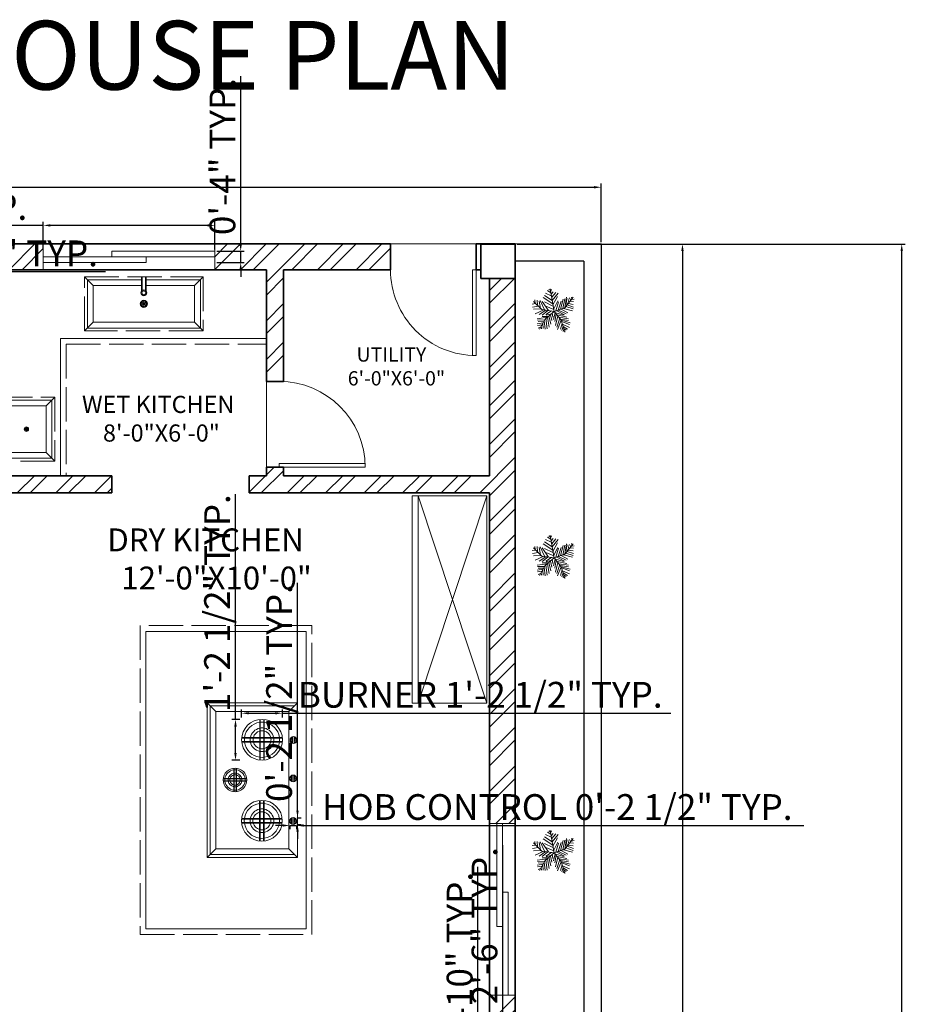
# Model space of a CAD drawing. Units: inches. Extents: x 889 to 1572, y 7262 to 8387.
# Tile 8 of 8: x 1263 to 1572, y 8007 to 8351. Entities that reach past the tile are written whole.
import ezdxf

# ---------------------------------------------------------------- set-up
doc = ezdxf.new("R2010")
doc.units = ezdxf.units.IN
doc.linetypes.add('ACAD_ISO02W100', pattern=[15, 12, -3])
for name, color, linetype, lineweight in [('A-ANNO-DIMS', 2, 'Continuous', 18), ('A-ANNO-TITL', 7, 'Continuous', 35), ('A-AREA-IDEN', 7, 'Continuous', 18), ('A-CASE-HIDN', 8, 'ACAD_ISO02W100', 13), ('A-DOOR', 4, 'Continuous', 18), ('A-EQPM', 8, 'Continuous', 18), ('A-FIXT-HIDN', 9, 'ACAD_ISO02W100', 13), ('A-FLOR-CASE', 8, 'Continuous', 20), ('A-FLOR-FIXT', 9, 'Continuous', 18), ('A-WALL', 7, 'Continuous', 35), ('A-WALL-PATT', 252, 'Continuous', 13), ('C-SITE', 7, 'Continuous', 30), ('L-PLNT', 94, 'Continuous', 13)]:
    doc.layers.add(name, color=color, linetype=linetype, lineweight=lineweight)
doc.layers.add('A-GLAZ', color=244, linetype='Continuous', lineweight=18, true_color=0x991b1e)
doc.styles.get("Standard").update_dxf_attribs({"font": 'arial.ttf'})
doc.dimstyles.new('ISO-25', dxfattribs={"dimtxt": 9, "dimasz": 2.5, "dimexe": 1.25, "dimexo": 0.625, "dimtad": 1, "dimlunit": 3, "dimtxsty": 'Standard', "dimcen": 2.5, "dimadec": 0, "dimazin": 0, "dimtfac": 1, "dimtmove": 0, "dimatfit": 3, "dimfxl": 1, "dimarcsym": 0})

# ---------------------------------------------------------------- blocks, each defined once
blk = doc.blocks.new('*U3')
for p, q in [((0, 0), (0, -6)), ((-40, 0), (-40, -6))]:
    blk.add_line(p, q)
blk.add_lwpolyline([(0, 0), (0, 40), (-1.75, 40), (-1.75, 0)], close=True)
blk.add_arc((0, 0), 40, 90, 180)
blk = doc.blocks.new('*U8')
for p, q in [((0, 0), (0, -6)), ((40, 0), (40, -6))]:
    blk.add_line(p, q)
blk.add_lwpolyline([(0, 0), (0, 40), (1.75, 40), (1.75, 0)], close=True)
blk.add_arc((0, 0), 40, 0, 90)
blk = doc.blocks.new('*U15')
for p, q in [((-8.737, 47.138), (-17.069, 52.711)), ((-10.186, 53.64), (-13.084, 55.962)), ((0, 0), (-10.5, 57)), ((-9.099, 51.782), (-6.563, 55.962)), ((-31.5, 4.5), (-52.5, 25.5)), ((-48.585, 21.131), (-49.309, 29.026)), ((-43.513, 28.561), (-42.427, 15.558)), ((-38.442, 26.239), (-34.819, 7.663)), ((-35.544, 28.097), (-24.314, 3.947)), ((-14.533, 2.09), (-30.834, 25.31)), ((-3.665, 19.273), (-27.574, 35.527)), ((-5.114, 28.097), (-24.676, 40.636)), ((-7.288, 39.707), (-21.778, 46.673)), ((-7.65, 43.423), (-2.578, 49.46)), ((-5.839, 35.992), (4.667, 48.067)), ((-5.114, 27.632), (10.463, 46.673)), ((-2.941, 16.486), (8.652, 37.85)), ((-1.129, 6.734), (9.014, 26.704)), ((10.101, 3.483), (17.708, 26.239)), ((16.259, 5.805), (23.142, 31.348)), ((22.055, 7.198), (27.489, 32.277)), ((27, 9), (48, 36)), ((27.127, 9.056), (31.112, 35.992)), ((31.836, 30.883), (32.561, 16.486)), ((35.096, 32.741), (37.27, 22.524)), ((38.719, 34.134), (41.979, 28.561)), ((40.53, 25.775), (48.862, 24.846)), ((43.791, 29.954), (51.036, 30.883)), ((44.153, 36.456), (45.239, 32.741)), ((-47.498, 19.737), (-55.83, 18.344)), ((-40.615, 13.7), (-55.105, 10.913)), ((-33.37, 6.269), (-52.207, 5.34)), ((-28.299, 3.483), (-47.86, -5.805)), ((-21.416, 3.018), (-38.079, -8.128)), ((0, 0), (-31.5, 4.5)), ((-15.982, 2.09), (-30.11, -9.521)), ((-24.314, 23.917), (-2.941, 13.7)), ((0, 0), (-22.5, -19.5)), ((-6.563, 1.161), (-21.416, -8.128)), ((-20.691, 13.7), (-1.129, 4.876)), ((0, 0), (27, 9)), ((0, 0), (18, -22.5)), ((3.942, 1.625), (11.187, 24.381)), ((6.478, 1.625), (26.04, -8.592)), ((11.187, 3.483), (30.749, -5.805)), ((18.07, 5.805), (35.096, -3.483)), ((24.229, 7.663), (46.688, 1.625)), ((29.662, 12.307), (48.137, 6.269)), ((33.285, 16.486), (48.862, 10.913)), ((36.183, 19.737), (48.137, 17.88)), ((-17.431, -15.094), (-42.789, -18.809)), ((-24.314, -21.596), (-42.427, -22.06)), ((-22.5, -19.5), (-37.5, -45)), ((-15.257, -12.772), (-30.11, -12.772)), ((-25.038, -23.918), (-22.865, -45.281)), ((-20.691, -18.345), (-17.793, -44.352)), ((-6.563, -5.805), (-19.967, -9.985)), ((-17.069, -15.094), (-12.721, -40.172)), ((-13.446, -11.378), (-8.737, -32.741)), ((-9.461, -8.592), (-6.201, -23.453)), ((-4.752, -3.483), (-3.665, -14.629)), ((2.493, -3.019), (-1.491, -20.202)), ((1.769, -2.555), (24.229, -9.521)), ((5.029, -6.27), (2.131, -25.775)), ((9.014, -11.378), (3.58, -35.992)), ((14.085, -16.951), (6.478, -40.172)), ((7.565, -9.056), (32.198, -14.629)), ((18.07, -22.524), (8.289, -45.745)), ((12.274, -15.094), (36.907, -18.809)), ((16.259, -19.738), (36.183, -22.989)), ((18, -22.5), (27, -52.5)), ((18.433, -22.524), (40.53, -29.026)), ((-28.299, -29.026), (-42.789, -31.348)), ((-30.834, -34.135), (-42.427, -35.528)), ((-34.457, -39.708), (-40.978, -42.494)), ((-26.849, -26.24), (-40.253, -25.775)), ((-32.646, -36.921), (-31.921, -44.352)), ((-29.023, -30.884), (-27.936, -43.887)), ((20.244, -30.419), (15.897, -44.816)), ((19.157, -25.311), (38.719, -33.206)), ((22.78, -37.85), (19.519, -48.532)), ((21.331, -32.741), (39.081, -40.636)), ((22.78, -38.314), (34.372, -44.816)), ((24.591, -45.745), (23.142, -50.854)), ((24.591, -43.423), (30.749, -47.603)), ((26.764, -49.925), (28.213, -50.854))]:
    blk.add_line(p, q)
blk = doc.blocks.new('*D28')
at = {"layer": 'A-ANNO-DIMS', "color": 0, "lineweight": -2, "transparency": 16777216}
for p, q in [((986.05, 8273.36), (986.05, 8293.82)), ((1466.05, 8273.36), (1466.05, 8293.82)), ((988.55, 8292.57), (1463.55, 8292.57))]:
    blk.add_line(p, q, dxfattribs=at)
at = {"layer": 'A-ANNO-DIMS', "color": 0, "transparency": 16777216}
for points in [[(988.55, 8292.98), (988.55, 8292.15), (986.05, 8292.57)], [(1463.55, 8292.98), (1463.55, 8292.15), (1466.05, 8292.57)]]:
    blk.add_solid(points, dxfattribs=at)
at = {"layer": 'Defpoints', "color": 0, "transparency": 16777216}
for p in [(1466.05, 8292.57), (986.05, 8272.73), (1466.05, 8272.73)]:
    blk.add_point(p, dxfattribs=at)
at = {"layer": 'A-ANNO-DIMS', "color": 0, "transparency": 16777216, "insert": (1226.05, 8297.79), "char_height": 9, "attachment_point": 5}
blk.add_mtext("40'", dxfattribs=at)
blk = doc.blocks.new('*D29')
at = {"layer": 'A-ANNO-DIMS', "color": 0, "lineweight": -2, "transparency": 16777216}
for p, q in [((1466.67, 8272.73), (1495.73, 8272.73)), ((1494.48, 8270.23), (1494.48, 7396.23)), ((1466.67, 7393.73), (1495.73, 7393.73))]:
    blk.add_line(p, q, dxfattribs=at)
at = {"layer": 'A-ANNO-DIMS', "color": 0, "transparency": 16777216}
for points in [[(1494.06, 8270.23), (1494.9, 8270.23), (1494.48, 8272.73)], [(1494.06, 7396.23), (1494.9, 7396.23), (1494.48, 7393.73)]]:
    blk.add_solid(points, dxfattribs=at)
at = {"layer": 'Defpoints', "color": 0, "transparency": 16777216}
for p in [(1466.05, 8272.73), (1466.05, 7393.73), (1494.48, 7393.73)]:
    blk.add_point(p, dxfattribs=at)
at = {"layer": 'A-ANNO-DIMS', "color": 0, "transparency": 16777216, "insert": (1489.26, 7833.23), "char_height": 9, "attachment_point": 5, "rotation": 90}
blk.add_mtext('73\'-3"', dxfattribs=at)
blk = doc.blocks.new('COOKTOP-BURNER-LARGE')
for p, q in [((6.34, 14.23), (6.34, 0.05)), ((6.54, 14.25), (6.54, 7.94)), ((7.74, 14.25), (7.74, 7.94)), ((7.94, 14.23), (7.94, 0.05)), ((0.03, 7.74), (6.34, 7.74)), ((0.05, 7.94), (14.23, 7.94)), ((6.54, 7.74), (6.54, 6.54)), ((6.54, 7.74), (7.74, 7.74)), ((7.74, 7.74), (7.74, 6.54)), ((7.94, 7.74), (14.25, 7.74)), ((0.03, 6.54), (6.34, 6.54)), ((0.05, 6.34), (14.23, 6.34)), ((6.54, 6.54), (7.74, 6.54)), ((6.54, 6.34), (6.54, 0.03)), ((7.74, 6.34), (7.74, 0.03)), ((7.94, 6.54), (14.25, 6.54))]:
    blk.add_line(p, q)
blk.add_circle((7.14, 7.14), 7.14)
for radius, start, end in [(6.14, 97.4895, 172.5105), (4.14, 101.1483, 168.8517), (6.14, 84.3899, 95.6101), (4.14, 81.662, 98.338), (6.14, 7.4895, 82.5105), (4.14, 11.1483, 78.8517), (6.14, 174.3899, 185.6101), (4.14, 171.662, 188.338), (3.14, 168.9754, 191.0246), (3.14, 104.772, 165.228), (3.14, 78.9754, 101.0246), (3.14, 14.772, 75.228), (3.14, 348.9754, 11.0246), (4.14, 351.662, 8.338), (6.14, 354.3899, 5.6101), (6.14, 187.4895, 262.5105), (4.14, 191.1483, 258.8517), (3.14, 194.772, 255.228), (3.14, 258.9754, 281.0246), (3.14, 284.772, 345.228), (4.14, 281.1483, 348.8517), (6.14, 277.4895, 352.5105), (4.14, 261.662, 278.338), (6.14, 264.3899, 275.6101)]:
    blk.add_arc((7.14, 7.14), radius, start, end)
blk = doc.blocks.new('COOKTOP-CONTROL')
for p, q in [((0.89, 2.34), (0.89, 0.04)), ((1.49, 2.34), (1.49, 0.04))]:
    blk.add_line(p, q)
blk.add_circle((1.19, 1.19), 1.19)
for radius, start, end in [(0.987, 107.6863, 252.3137), (0.587, 120.7077, 239.2923), (0.387, 140.7361, 219.2639), (0.987, 287.6863, 72.3137), (0.587, 300.7077, 59.2923), (0.387, 320.7361, 39.2639)]:
    blk.add_arc((1.19, 1.19), radius, start, end)
blk = doc.blocks.new('GLAZ-SLIDER-60IN')
for p, q in [((0, 60), (0, 24)), ((2, 60), (2, 0)), ((2, 36), (4, 36)), ((4, 36), (4, 0)), ((2, 24), (0, 24))]:
    blk.add_line(p, q)
blk = doc.blocks.new('*D37')
at = {"layer": 'A-ANNO-DIMS', "color": 0, "lineweight": -2, "transparency": 16777216}
for p, q in [((1271.05, 8279.23), (1163.57, 8279.23)), ((1271.05, 8270.86), (1271.05, 8280.48)), ((1328.55, 8279.23), (1273.55, 8279.23)), ((1331.05, 8270.86), (1331.05, 8280.48))]:
    blk.add_line(p, q, dxfattribs=at)
at = {"layer": 'A-ANNO-DIMS', "color": 0, "transparency": 16777216}
for points in [[(1273.55, 8279.65), (1273.55, 8278.81), (1271.05, 8279.23)], [(1328.55, 8279.65), (1328.55, 8278.81), (1331.05, 8279.23)]]:
    blk.add_solid(points, dxfattribs=at)
at = {"layer": 'Defpoints', "color": 0, "transparency": 16777216}
for p in [(1271.05, 8279.23), (1271.05, 8270.23), (1331.05, 8270.23)]:
    blk.add_point(p, dxfattribs=at)
at = {"layer": 'A-ANNO-DIMS', "color": 0, "transparency": 16777216, "insert": (1216.06, 8284.51), "char_height": 9, "attachment_point": 5}
blk.add_mtext('SLIDER 5\'-0" TYP.', dxfattribs=at)
blk = doc.blocks.new('*D38')
at = {"layer": 'A-ANNO-DIMS', "color": 0, "lineweight": -2, "transparency": 16777216}
for p, q in [((1340.05, 8272.73), (1340.05, 8331.34)), ((1331.67, 8270.23), (1341.3, 8270.23)), ((1340.05, 8266.23), (1340.05, 8270.23)), ((1331.67, 8266.23), (1341.3, 8266.23)), ((1340.05, 8263.73), (1340.05, 8261.23))]:
    blk.add_line(p, q, dxfattribs=at)
at = {"layer": 'A-ANNO-DIMS', "color": 0, "transparency": 16777216}
for points in [[(1339.63, 8272.73), (1340.47, 8272.73), (1340.05, 8270.23)], [(1339.63, 8263.73), (1340.47, 8263.73), (1340.05, 8266.23)]]:
    blk.add_solid(points, dxfattribs=at)
at = {"layer": 'Defpoints', "color": 0, "transparency": 16777216}
for p in [(1331.05, 8270.23), (1340.05, 8270.23), (1331.05, 8266.23)]:
    blk.add_point(p, dxfattribs=at)
at = {"layer": 'A-ANNO-DIMS', "color": 0, "transparency": 16777216, "insert": (1334.83, 8303.29), "char_height": 9, "attachment_point": 5, "rotation": 90}
blk.add_mtext('0\'-4" TYP.', dxfattribs=at)
blk = doc.blocks.new('*D41')
at = {"layer": 'A-ANNO-DIMS', "color": 0, "lineweight": -2, "transparency": 16777216}
for p, q in [((1175.74, 8265.61), (1175.74, 8261.83)), ((1196.74, 8265.61), (1196.74, 8261.83)), ((1178.24, 8263.08), (1194.24, 8263.08)), ((1196.74, 8263.08), (1292.84, 8263.08))]:
    blk.add_line(p, q, dxfattribs=at)
at = {"layer": 'A-ANNO-DIMS', "color": 0, "transparency": 16777216}
for points in [[(1178.24, 8263.5), (1178.24, 8262.66), (1175.74, 8263.08)], [(1194.24, 8263.5), (1194.24, 8262.66), (1196.74, 8263.08)]]:
    blk.add_solid(points, dxfattribs=at)
at = {"layer": 'Defpoints', "color": 0, "transparency": 16777216}
for p in [(1175.74, 8266.23), (1196.74, 8266.23), (1196.74, 8263.08)]:
    blk.add_point(p, dxfattribs=at)
at = {"layer": 'A-ANNO-DIMS', "color": 0, "transparency": 16777216, "insert": (1246.04, 8268.3), "char_height": 9, "attachment_point": 5}
blk.add_mtext('VENT 1\'-9" TYP.', dxfattribs=at)
blk = doc.blocks.new('*D48')
at = {"layer": 'A-ANNO-DIMS', "color": 0, "lineweight": -2, "transparency": 16777216}
for p, q in [((1431.66, 8003.87), (1431.66, 8062.63)), ((1426.67, 8003.87), (1432.91, 8003.87)), ((1431.66, 7976.19), (1431.66, 8001.37)), ((1426.67, 7973.69), (1432.91, 7973.69))]:
    blk.add_line(p, q, dxfattribs=at)
at = {"layer": 'A-ANNO-DIMS', "color": 0, "transparency": 16777216}
for points in [[(1431.24, 8001.37), (1432.07, 8001.37), (1431.66, 8003.87)], [(1431.24, 7976.19), (1432.07, 7976.19), (1431.66, 7973.69)]]:
    blk.add_solid(points, dxfattribs=at)
at = {"layer": 'Defpoints', "color": 0, "transparency": 16777216}
for p in [(1426.05, 8003.87), (1431.66, 8003.87), (1426.05, 7973.69)]:
    blk.add_point(p, dxfattribs=at)
at = {"layer": 'A-ANNO-DIMS', "color": 0, "transparency": 16777216, "insert": (1426.44, 8034.5), "char_height": 9, "attachment_point": 5, "rotation": 90}
blk.add_mtext('2\'-6" TYP.', dxfattribs=at)
blk = doc.blocks.new('*D55')
at = {"layer": 'A-ANNO-DIMS', "color": 0, "lineweight": -2, "transparency": 16777216}
for p, q in [((1354.69, 8069.51), (1352.19, 8069.51)), ((1357.19, 8069.51), (1359.56, 8069.51)), ((1357.19, 8069.25), (1357.19, 8068.26)), ((1359.56, 8069.25), (1359.56, 8068.26)), ((1362.06, 8069.51), (1536.86, 8069.51))]:
    blk.add_line(p, q, dxfattribs=at)
at = {"layer": 'A-ANNO-DIMS', "color": 0, "transparency": 16777216}
for points in [[(1354.69, 8069.93), (1354.69, 8069.1), (1357.19, 8069.51)], [(1362.06, 8069.93), (1362.06, 8069.1), (1359.56, 8069.51)]]:
    blk.add_solid(points, dxfattribs=at)
at = {"layer": 'Defpoints', "color": 0, "transparency": 16777216}
for p in [(1357.19, 8069.87), (1359.56, 8069.87), (1359.56, 8069.51)]:
    blk.add_point(p, dxfattribs=at)
at = {"layer": 'A-ANNO-DIMS', "color": 0, "transparency": 16777216, "insert": (1450.71, 8074.8), "char_height": 9, "attachment_point": 5}
blk.add_mtext('HOB CONTROL 0\'-2 1/2" TYP.', dxfattribs=at)
blk = doc.blocks.new('*D56')
at = {"layer": 'A-ANNO-DIMS', "color": 0, "lineweight": -2, "transparency": 16777216}
for p, q in [((1359.92, 8074.75), (1359.92, 8154.33)), ((1359.92, 8069.87), (1359.92, 8072.25)), ((1360.19, 8072.25), (1361.17, 8072.25)), ((1360.19, 8069.87), (1361.17, 8069.87)), ((1359.92, 8067.37), (1359.92, 8064.87))]:
    blk.add_line(p, q, dxfattribs=at)
at = {"layer": 'A-ANNO-DIMS', "color": 0, "transparency": 16777216}
for points in [[(1359.5, 8074.75), (1360.33, 8074.75), (1359.92, 8072.25)], [(1359.5, 8067.37), (1360.33, 8067.37), (1359.92, 8069.87)]]:
    blk.add_solid(points, dxfattribs=at)
at = {"layer": 'Defpoints', "color": 0, "transparency": 16777216}
for p in [(1359.56, 8072.25), (1359.56, 8069.87), (1359.92, 8072.25)]:
    blk.add_point(p, dxfattribs=at)
at = {"layer": 'A-ANNO-DIMS', "color": 0, "transparency": 16777216, "insert": (1354.64, 8115.79), "char_height": 9, "attachment_point": 5, "rotation": 90}
blk.add_mtext('0\'-2 1/2" TYP.', dxfattribs=at)
blk = doc.blocks.new('*D57')
at = {"layer": 'A-ANNO-DIMS', "color": 0, "lineweight": -2, "transparency": 16777216}
for p, q in [((1422.97, 7957.73), (1422.97, 8055.08)), ((1418.49, 7957.73), (1424.22, 7957.73)), ((1422.97, 7926.23), (1422.97, 7955.23)), ((1418.49, 7923.73), (1424.22, 7923.73))]:
    blk.add_line(p, q, dxfattribs=at)
at = {"layer": 'A-ANNO-DIMS', "color": 0, "transparency": 16777216}
for points in [[(1422.55, 7955.23), (1423.38, 7955.23), (1422.97, 7957.73)], [(1422.55, 7926.23), (1423.38, 7926.23), (1422.97, 7923.73)]]:
    blk.add_solid(points, dxfattribs=at)
at = {"layer": 'Defpoints', "color": 0, "transparency": 16777216}
for p in [(1417.87, 7957.73), (1422.97, 7957.73), (1417.87, 7923.73)]:
    blk.add_point(p, dxfattribs=at)
at = {"layer": 'A-ANNO-DIMS', "color": 0, "transparency": 16777216, "insert": (1417.74, 8007.65), "char_height": 9, "attachment_point": 5, "rotation": 90}
blk.add_mtext('BIKE 2\'-10" TYP.', dxfattribs=at)
blk = doc.blocks.new('*D61')
at = {"layer": 'A-ANNO-DIMS', "color": 0, "lineweight": -2, "transparency": 16777216}
for p, q in [((1340.38, 8107.23), (1340.38, 8110)), ((1342.88, 8108.75), (1352.15, 8108.75)), ((1354.65, 8107.23), (1354.65, 8110)), ((1354.65, 8108.75), (1490.42, 8108.75))]:
    blk.add_line(p, q, dxfattribs=at)
at = {"layer": 'A-ANNO-DIMS', "color": 0, "transparency": 16777216}
for points in [[(1342.88, 8109.16), (1342.88, 8108.33), (1340.38, 8108.75)], [(1352.15, 8109.16), (1352.15, 8108.33), (1354.65, 8108.75)]]:
    blk.add_solid(points, dxfattribs=at)
at = {"layer": 'Defpoints', "color": 0, "transparency": 16777216}
for p in [(1354.65, 8108.75), (1340.38, 8106.61), (1354.65, 8106.61)]:
    blk.add_point(p, dxfattribs=at)
at = {"layer": 'A-ANNO-DIMS', "color": 0, "transparency": 16777216, "insert": (1423.78, 8114.03), "char_height": 9, "attachment_point": 5}
blk.add_mtext('BURNER 1\'-2 1/2" TYP.', dxfattribs=at)
blk = doc.blocks.new('*D62')
at = {"layer": 'A-ANNO-DIMS', "color": 0, "lineweight": -2, "transparency": 16777216}
for p, q in [((1338.24, 8106.61), (1338.24, 8185.34)), ((1339.75, 8106.61), (1336.99, 8106.61)), ((1338.24, 8094.83), (1338.24, 8104.11)), ((1339.75, 8092.33), (1336.99, 8092.33))]:
    blk.add_line(p, q, dxfattribs=at)
at = {"layer": 'A-ANNO-DIMS', "color": 0, "transparency": 16777216}
for points in [[(1337.82, 8104.11), (1338.65, 8104.11), (1338.24, 8106.61)], [(1337.82, 8094.83), (1338.65, 8094.83), (1338.24, 8092.33)]]:
    blk.add_solid(points, dxfattribs=at)
at = {"layer": 'Defpoints', "color": 0, "transparency": 16777216}
for p in [(1338.24, 8106.61), (1340.38, 8106.61), (1340.38, 8092.33)]:
    blk.add_point(p, dxfattribs=at)
at = {"layer": 'A-ANNO-DIMS', "color": 0, "transparency": 16777216, "insert": (1332.96, 8147.22), "char_height": 9, "attachment_point": 5, "rotation": 90}
blk.add_mtext('1\'-2 1/2" TYP.', dxfattribs=at)
blk = doc.blocks.new('*D70')
at = {"layer": 'A-ANNO-DIMS', "color": 0, "lineweight": -2, "transparency": 16777216}
for p, q in [((1436.67, 8272.73), (1572.38, 8272.73)), ((1571.13, 7585.23), (1571.13, 8270.23)), ((1436.67, 7582.73), (1572.38, 7582.73))]:
    blk.add_line(p, q, dxfattribs=at)
at = {"layer": 'A-ANNO-DIMS', "color": 0, "transparency": 16777216}
for points in [[(1570.71, 8270.23), (1571.54, 8270.23), (1571.13, 8272.73)], [(1570.71, 7585.23), (1571.54, 7585.23), (1571.13, 7582.73)]]:
    blk.add_solid(points, dxfattribs=at)
at = {"layer": 'Defpoints', "color": 0, "transparency": 16777216}
for p in [(1436.05, 8272.73), (1571.13, 8272.73), (1436.05, 7582.73)]:
    blk.add_point(p, dxfattribs=at)
at = {"layer": 'A-ANNO-DIMS', "color": 0, "transparency": 16777216, "insert": (1565.91, 7927.73), "char_height": 9, "attachment_point": 5, "rotation": 90}
blk.add_mtext('57\'-6"', dxfattribs=at)
blk = doc.blocks.new('*D74')
at = {"layer": 'A-ANNO-DIMS', "color": 0, "lineweight": -2, "transparency": 16777216}
for p, q in [((1247.05, 8161.11), (1247.05, 7262.35)), ((1253.05, 8161.11), (1253.05, 7262.35)), ((1244.55, 7263.6), (1242.05, 7263.6)), ((1247.05, 7263.6), (1253.05, 7263.6)), ((1255.55, 7263.6), (1283.22, 7263.6))]:
    blk.add_line(p, q, dxfattribs=at)
at = {"layer": 'A-ANNO-DIMS', "color": 0, "transparency": 16777216}
for points in [[(1244.55, 7264.02), (1244.55, 7263.19), (1247.05, 7263.6)], [(1255.55, 7264.02), (1255.55, 7263.19), (1253.05, 7263.6)]]:
    blk.add_solid(points, dxfattribs=at)
at = {"layer": 'Defpoints', "color": 0, "transparency": 16777216}
for p in [(1247.05, 8161.73), (1253.05, 8161.73), (1253.05, 7263.6)]:
    blk.add_point(p, dxfattribs=at)
at = {"layer": 'A-ANNO-DIMS', "color": 0, "transparency": 16777216, "insert": (1270.64, 7268.82), "char_height": 9, "attachment_point": 5}
blk.add_mtext('0\'-6"', dxfattribs=at)

msp = doc.modelspace()

# ---------------------------------------------------------------- hatches: boundary and pattern name
at = {"layer": 'A-WALL-PATT'}
h = msp.add_hatch(dxfattribs=at)
h.set_pattern_fill('ANSI32', color=256)
h.paths.add_polyline_path([(1166.049, 7624.731), (1163.049, 7624.731), (1163.049, 7774.731), (1154.049, 7774.731), (1154.049, 7768.731), (1157.049, 7768.731), (1157.049, 7624.731), (1106.049, 7624.731), (1106.049, 7615.731), (1166.049, 7615.731), (1166.049, 7618.431)])
h.paths.add_polyline_path([(1025.049, 7666.731), (1016.049, 7666.731), (1016.049, 7615.731), (1076.049, 7615.731), (1076.049, 7624.731), (1025.049, 7624.731)])
h.paths.add_polyline_path([(1025.049, 7768.731), (1118.049, 7768.731), (1118.049, 7774.731), (1025.049, 7774.731), (1025.049, 7897.731), (1115.049, 7897.731), (1115.049, 7906.731), (1109.049, 7906.731), (1109.049, 7903.731), (1025.049, 7903.731), (1025.049, 7923.231), (1016.049, 7923.231), (1016.049, 7726.731), (1025.049, 7726.731)])
h.paths.add_polyline_path([(1436.049, 7897.731), (1427.049, 7897.731), (1427.049, 7883.374), (1436.049, 7883.374)])
h.paths.add_polyline_path([(1436.049, 7853.374), (1427.049, 7853.374), (1427.049, 7843.731), (1415.049, 7843.731), (1415.049, 7837.731), (1427.049, 7837.731), (1427.049, 7831.731), (1436.049, 7831.731)])
h.paths.add_polyline_path([(1436.049, 8010.183), (1427.049, 8010.183), (1427.049, 7970.456), (1370.049, 7970.456), (1370.049, 7963.731), (1427.049, 7963.731), (1427.049, 7957.731), (1436.049, 7957.731)])
h.paths.add_polyline_path([(1436.049, 7747.731), (1427.049, 7747.731), (1427.049, 7741.731), (1344.721, 7741.731), (1344.721, 7735.731), (1349.049, 7735.731), (1349.049, 7672.731), (1355.049, 7672.731), (1355.049, 7735.731), (1427.049, 7735.731), (1427.049, 7721.931), (1436.049, 7721.931)])
h.paths.add_polyline_path([(1436.049, 7700.931), (1427.049, 7700.931), (1427.049, 7591.731), (1355.049, 7591.731), (1355.049, 7642.731), (1349.049, 7642.731), (1349.049, 7591.731), (1310.049, 7591.731), (1310.049, 7582.731), (1436.049, 7582.731)])
h.paths.add_polyline_path([(1392.42, 8272.731), (1331.049, 8272.731), (1331.049, 8263.731), (1349.049, 8263.731), (1349.049, 8224.731), (1355.049, 8224.731), (1355.049, 8263.731), (1392.42, 8263.731)])
h.paths.add_polyline_path([(1271.049, 8272.731), (1196.736, 8272.731), (1196.736, 8263.731), (1247.049, 8263.731), (1247.049, 8203.731), (1244.049, 8203.731), (1244.049, 8197.731), (1247.049, 8197.731), (1247.049, 8161.731), (1253.049, 8161.731), (1253.049, 8185.731), (1295.049, 8185.731), (1295.049, 8191.731), (1253.049, 8191.731), (1253.049, 8263.731), (1271.049, 8263.731)])
h.paths.add_polyline_path([(1175.736, 8272.731), (1102.037, 8272.731), (1102.037, 8263.731), (1157.049, 8263.731), (1157.049, 8158.731), (1163.049, 8158.731), (1163.049, 8197.731), (1214.049, 8197.731), (1214.049, 8203.731), (1163.049, 8203.731), (1163.049, 8263.731), (1175.736, 8263.731)])
h.paths.add_polyline_path([(1072.037, 8272.731), (1016.049, 8272.731), (1016.049, 8221.731), (1025.049, 8221.731), (1025.049, 8263.731), (1072.037, 8263.731)])
h.paths.add_polyline_path([(1163.049, 8122.731), (1157.049, 8122.731), (1157.049, 8119.731), (1025.049, 8119.731), (1025.049, 8161.731), (1016.049, 8161.731), (1016.049, 8071.731), (1025.049, 8071.731), (1025.049, 8113.731), (1157.049, 8113.731), (1157.049, 8110.731), (1163.049, 8110.731)])
h.paths.add_polyline_path([(1025.049, 8011.731), (1016.049, 8011.731), (1016.049, 7944.231), (1025.049, 7944.231), (1025.049, 7963.731), (1109.049, 7963.731), (1109.049, 7936.731), (1115.049, 7936.731), (1115.049, 7963.731), (1163.049, 7963.731), (1163.049, 8074.731), (1157.049, 8074.731), (1157.049, 7969.731), (1025.049, 7969.731)])
h.paths.add_polyline_path([(1314.721, 7741.731), (1307.049, 7741.731), (1307.049, 7837.731), (1319.049, 7837.731), (1319.049, 7843.731), (1307.049, 7843.731), (1307.049, 7963.731), (1310.049, 7963.731), (1310.049, 7970.456), (1301.049, 7970.456), (1301.049, 7837.731), (1301.049, 7741.731), (1250.049, 7741.731), (1250.049, 7735.731), (1314.721, 7735.731)])
h.paths.add_polyline_path([(1211.049, 7735.731), (1214.049, 7735.731), (1214.049, 7741.731), (1205.049, 7741.731), (1205.049, 7624.731), (1202.049, 7624.731), (1202.049, 7615.731), (1205.049, 7615.731), (1205.049, 7582.731), (1250.049, 7582.731), (1250.049, 7591.731), (1211.049, 7591.731)])
h.paths.add_polyline_path([(1436.049, 8260.718), (1427.049, 8260.718), (1427.049, 8191.731), (1355.049, 8191.731), (1355.049, 8194.731), (1349.049, 8194.731), (1349.049, 8191.731), (1343.049, 8191.731), (1343.049, 8185.731), (1427.049, 8185.731), (1427.049, 8070.183), (1436.049, 8070.183)])

# ---------------------------------------------------------------- linework, layer by layer
at = {"layer": 'A-CASE-HIDN'}
for q in [(1349.049, 8237.731), (1279.049, 8191.731)]:
    msp.add_line((1279.049, 8237.731), q, dxfattribs=at)
msp.add_lwpolyline([(1364.909, 8139.364), (1304.909, 8139.364), (1304.909, 8031.364), (1364.909, 8031.364)], close=True, dxfattribs=at)
at = {"layer": 'A-DOOR'}
for p, q in [((1422.42, 8272.731), (1392.42, 8272.731)), ((1349.049, 8224.731), (1349.049, 8194.731))]:
    msp.add_line(p, q, dxfattribs=at)
at = {"layer": 'A-EQPM'}
for p, q in [((1331.371, 8109.364), (1328.371, 8112.364)), ((1356.909, 8109.364), (1359.909, 8112.364)), ((1337.615, 8089.547), (1337.615, 8081.324)), ((1337.731, 8089.558), (1337.731, 8085.899)), ((1338.426, 8089.558), (1338.426, 8085.899)), ((1338.542, 8089.547), (1338.542, 8081.324)), ((1333.956, 8085.783), (1337.615, 8085.783)), ((1333.956, 8085.088), (1337.615, 8085.088)), ((1333.967, 8085.899), (1342.19, 8085.899)), ((1333.967, 8084.972), (1342.19, 8084.972)), ((1337.731, 8085.783), (1337.731, 8085.088)), ((1337.731, 8085.783), (1338.426, 8085.783)), ((1337.731, 8085.088), (1338.426, 8085.088)), ((1337.731, 8084.972), (1337.731, 8081.313)), ((1338.426, 8085.783), (1338.426, 8085.088)), ((1338.426, 8084.972), (1338.426, 8081.313)), ((1338.542, 8085.783), (1342.201, 8085.783)), ((1338.542, 8085.088), (1342.201, 8085.088)), ((1331.371, 8061.364), (1328.371, 8058.364)), ((1356.909, 8061.364), (1359.909, 8058.364))]:
    msp.add_line(p, q, dxfattribs=at)
for points in [[(1359.909, 8112.364), (1328.371, 8112.364), (1328.371, 8058.364), (1359.909, 8058.364)], [(1356.909, 8109.364), (1331.371, 8109.364), (1331.371, 8061.364), (1356.909, 8061.364)]]:
    msp.add_lwpolyline(points, close=True, dxfattribs=at)
msp.add_lwpolyline([(1358.909, 8111.364), (1329.371, 8111.364), (1329.371, 8059.364), (1358.909, 8059.364)], dxfattribs=at)
msp.add_circle((1338.078, 8085.436), 4.138, dxfattribs=at)
for radius, start, end in [(3.558, 97.48949, 172.51051), (2.399, 101.14831, 168.85169), (1.819, 104.77197, 165.22803), (3.558, 84.38991, 95.61009), (2.399, 81.66203, 98.33797), (1.819, 78.97545, 101.02455), (3.558, 7.48949, 82.51051), (2.399, 11.14831, 78.85169), (1.819, 14.77197, 75.22803), (3.558, 174.38991, 185.61009), (3.558, 187.48949, 262.51051), (2.399, 171.66203, 188.33797), (2.399, 191.14831, 258.85169), (1.819, 168.97545, 191.02455), (1.819, 194.77197, 255.22803), (1.819, 258.97545, 281.02455), (2.399, 261.66203, 278.33797), (3.558, 277.48949, 352.51051), (2.399, 281.14831, 348.85169), (1.819, 284.77197, 345.22803), (1.819, 348.97545, 11.02455), (2.399, 351.66203, 8.33797), (3.558, 354.38991, 5.61009), (3.558, 264.38991, 275.61009)]:
    msp.add_arc((1338.078, 8085.436), radius, start, end, dxfattribs=at)
at = {"layer": 'A-FIXT-HIDN'}
for points in [[(1285.466, 8261.263), (1326.947, 8261.263), (1326.947, 8242.372), (1285.466, 8242.372)], [(1255.235, 8219.196), (1275.072, 8219.196), (1275.072, 8196.835), (1255.235, 8196.835)]]:
    msp.add_lwpolyline(points, close=True, dxfattribs=at)
at = {"layer": 'A-FLOR-CASE'}
for p, q in [((1277.049, 8239.731), (1349.049, 8239.731)), ((1277.049, 8239.731), (1277.049, 8191.731)), ((1400.049, 8184.731), (1426.049, 8184.731)), ((1400.049, 8184.731), (1400.049, 8112.214)), ((1402.049, 8184.731), (1402.049, 8112.214)), ((1426.049, 8184.731), (1402.049, 8112.214)), ((1426.049, 8112.214), (1402.049, 8184.731)), ((1426.049, 8184.731), (1426.049, 8112.214)), ((1426.049, 8112.214), (1400.049, 8112.214))]:
    msp.add_line(p, q, dxfattribs=at)
msp.add_lwpolyline([(1362.909, 8137.364), (1306.909, 8137.364), (1306.909, 8033.364), (1362.909, 8033.364)], close=True, dxfattribs=at)
at = {"layer": 'A-FLOR-FIXT'}
for p, q in [((1288.466, 8258.263), (1285.466, 8261.263)), ((1305.406, 8261.263), (1305.406, 8256.261)), ((1305.606, 8261.263), (1305.606, 8256.46)), ((1306.806, 8261.263), (1306.806, 8256.46)), ((1307.006, 8261.263), (1307.006, 8256.261)), ((1323.947, 8258.263), (1326.947, 8261.263)), ((1304.971, 8251.817), (1307.441, 8251.817)), ((1305.309, 8250.968), (1307.104, 8252.666)), ((1307.092, 8250.957), (1305.32, 8252.678)), ((1306.206, 8253.052), (1306.206, 8250.582)), ((1288.466, 8245.372), (1285.466, 8242.372)), ((1323.947, 8245.372), (1326.947, 8242.372)), ((1272.072, 8216.196), (1275.072, 8219.196)), ((1264.383, 8208.016), (1265.924, 8208.016)), ((1264.618, 8207.462), (1265.689, 8208.57)), ((1265.677, 8207.451), (1264.63, 8208.581)), ((1265.154, 8208.786), (1265.154, 8207.245)), ((1272.072, 8199.835), (1275.072, 8196.835))]:
    msp.add_line(p, q, dxfattribs=at)
for points in [[(1307.006, 8260.263), (1325.947, 8260.263), (1325.947, 8243.372), (1286.466, 8243.372), (1286.466, 8260.263), (1305.406, 8260.263)], [(1307.006, 8258.263), (1323.947, 8258.263), (1323.947, 8245.372), (1288.466, 8245.372), (1288.466, 8258.263), (1305.406, 8258.263)], [(1256.235, 8208.616), (1256.235, 8218.196), (1274.072, 8218.196), (1274.072, 8197.835), (1256.235, 8197.835), (1256.235, 8207.416)], [(1258.235, 8208.616), (1258.235, 8216.196), (1272.072, 8216.196), (1272.072, 8199.835), (1258.235, 8199.835), (1258.235, 8207.416)]]:
    msp.add_lwpolyline(points, dxfattribs=at)
for centre, radius in [((1306.206, 8255.658), 1.002), ((1306.206, 8255.658), 0.702), ((1306.206, 8251.817), 1.235), ((1306.206, 8251.817), 1.035), ((1265.154, 8208.016), 0.771), ((1265.154, 8208.016), 0.471)]:
    msp.add_circle(centre, radius, dxfattribs=at)
at = {"layer": 'A-GLAZ'}
for points in [[(1331.049, 8272.731), (1331.049, 8263.731), (1271.049, 8263.731), (1271.049, 8272.731)], [(1427.049, 8070.183), (1436.049, 8070.183), (1436.049, 8010.183), (1427.049, 8010.183)]]:
    msp.add_lwpolyline(points, close=True, dxfattribs=at)
at = {"layer": 'A-WALL'}
for p, q in [((1016.049, 8272.731), (1392.42, 8272.731)), ((1392.42, 8272.731), (1392.42, 8263.731)), ((1422.42, 8272.731), (1422.42, 8263.731)), ((1422.42, 8272.731), (1436.049, 8272.731)), ((1427.049, 8272.718), (1427.049, 8272.731)), ((1436.049, 8272.731), (1436.049, 7582.731)), ((1253.049, 8263.731), (1349.049, 8263.731)), ((1349.049, 8263.731), (1349.049, 8224.731)), ((1355.049, 8263.731), (1355.049, 8224.731)), ((1355.049, 8263.731), (1392.42, 8263.731)), ((1422.42, 8263.731), (1424.049, 8263.731)), ((1427.049, 8260.718), (1427.049, 8191.731)), ((1355.049, 8224.731), (1349.049, 8224.731)), ((1355.049, 8194.731), (1349.049, 8194.731)), ((1349.049, 8194.731), (1349.049, 8191.731)), ((1355.049, 8194.731), (1355.049, 8191.731)), ((1253.049, 8191.731), (1295.049, 8191.731)), ((1295.049, 8191.731), (1295.049, 8185.731)), ((1343.049, 8191.731), (1349.049, 8191.731)), ((1343.049, 8191.731), (1343.049, 8185.731)), ((1355.049, 8191.731), (1427.049, 8191.731)), ((1253.049, 8185.731), (1295.049, 8185.731)), ((1343.049, 8185.731), (1427.049, 8185.731)), ((1427.049, 8185.731), (1427.049, 7970.456))]:
    msp.add_line(p, q, dxfattribs=at)
msp.add_lwpolyline([(1424.049, 8272.718), (1436.049, 8272.718), (1436.049, 8260.718), (1424.049, 8260.718)], close=True, dxfattribs=at)
at = {"layer": 'C-SITE'}
for p, q in [((1466.049, 8272.731), (1436.049, 8272.718)), ((1460.049, 8272.731), (1460.049, 8272.729)), ((1466.049, 8272.731), (1466.049, 7582.731)), ((1460.049, 8266.729), (1436.051, 8266.718)), ((1460.049, 8266.729), (1460.049, 7582.731)), ((1466.051, 8266.731), (1466.049, 8266.731))]:
    msp.add_line(p, q, dxfattribs=at)

# ---------------------------------------------------------------- block references
at = {"layer": 'A-DOOR', "xscale": 0.75, "yscale": 0.75, "zscale": 0.75}
for name, p, rotation in [('*U8', (1422.42, 8263.731), 180.0000000000077), ('*U3', (1353.549, 8194.731), 270.0000000000077)]:
    msp.add_blockref(name, p, dxfattribs=dict(at, rotation=rotation))
at = {"layer": 'A-EQPM'}
for name, p in [('COOKTOP-BURNER-LARGE', (1340.376, 8092.331)), ('COOKTOP-CONTROL', (1357.292, 8098.183)), ('COOKTOP-CONTROL', (1357.186, 8084.777)), ('COOKTOP-CONTROL', (1357.186, 8069.871))]:
    msp.add_blockref(name, p, dxfattribs=at)
at = {"layer": 'A-EQPM', "rotation": 180}
msp.add_blockref('COOKTOP-BURNER-LARGE', (1354.598, 8078.295), dxfattribs=at)
at = {"layer": 'A-GLAZ'}
for p, rotation in [((1331.049, 8266.232), 89.99999999999666), ((1433.548, 8070.184), 180)]:
    msp.add_blockref('GLAZ-SLIDER-60IN', p, dxfattribs=dict(at, rotation=rotation))
at = {"layer": 'L-PLNT', "xscale": 0.137481440781912, "yscale": 0.137481440781912, "zscale": 0.137481440781912}
for p in [(1449.619, 8249.178), (1449.619, 8163.045), (1449.619, 8059.968)]:
    msp.add_blockref('*U15', p, dxfattribs=at)

# ---------------------------------------------------------------- texts
at = {"layer": 'A-ANNO-TITL', "insert": (978.629, 8350.694), "char_height": 24, "attachment_point": 1}
msp.add_mtext_dynamic_manual_height_columns('GROUND FLOOR HOUSE PLAN', width=625.16453, gutter_width=0, heights=[25.177], dxfattribs=at)
at = {"layer": 'A-AREA-IDEN', "attachment_point": 1}
for s, width, insert, char_height in [('  UTILITY\\P6\'-0"X6\'-0"', 32.40356, (1377.479, 8236.625), 5), ('WET KITCHEN\\P    8\'-0"X6\'-0"', 59.61764, (1284.581, 8219.675), 6), ('DRY KITCHEN\\P  12\'-0"X10\'-0"', 75.12166, (1293.426, 8173.331), 8)]:
    msp.add_mtext_dynamic_manual_height_columns(s, width=width, gutter_width=12.5, heights=[0], dxfattribs=dict(at, insert=insert, char_height=char_height))

# ---------------------------------------------------------------- dimensions: what is measured, and where the dimension line sits
at = {"layer": 'A-ANNO-DIMS'}
for base, p1, p2, angle, text, picture, middle in [((1340.049, 8270.231), (1331.049, 8266.231), (1331.049, 8270.231), 90, '<> TYP.', '*D38', (1334.828, 8303.286)), ((1271.049, 8279.231), (1331.049, 8270.231), (1271.049, 8270.231), 180, 'SLIDER <> TYP.', '*D37', (1216.06, 8284.51)), ((1338.235, 8106.606), (1340.376, 8092.331), (1340.376, 8106.606), 90, '<> TYP.', '*D62', (1332.957, 8147.223)), ((1359.917, 8072.246), (1359.561, 8069.871), (1359.561, 8072.246), 90, '<> TYP.', '*D56', (1354.638, 8115.786)), ((1431.658, 8003.866), (1426.049, 7973.694), (1426.049, 8003.866), 90, '<> TYP.', '*D48', (1426.437, 8034.497)), ((1422.965, 7957.731), (1417.865, 7923.731), (1417.865, 7957.731), 90, 'BIKE <> TYP.', '*D57', (1417.745, 8007.655))]:
    dim = msp.add_linear_dim(base=base, p1=p1, p2=p2, angle=angle, text=text, dimstyle='ISO-25', override={"dimdec": 1, "dimlfac": 1, "dimrnd": 0, "dimzin": 1, "dimdsep": 46, "dimlunit": 4, "dimfrac": 2}, dxfattribs=at)
    dim.commit()
    dim.dimension.update_dxf_attribs({"geometry": picture, "text_midpoint": middle})
for base, p1, p2, override, picture, middle in [((1466.049, 8292.566), (986.049, 8272.731), (1466.049, 8272.731), {"dimclrd": 0, "dimclre": 0, "dimclrt": 0}, '*D28', (1226.049, 8297.786)), ((1253.049, 7263.604), (1247.049, 8161.731), (1253.049, 8161.731), {"dimdec": 1, "dimlfac": 1, "dimrnd": 0, "dimzin": 1, "dimdsep": 46, "dimlunit": 4, "dimfrac": 2}, '*D74', (1270.636, 7268.824))]:
    dim = msp.add_linear_dim(base=base, p1=p1, p2=p2, dimstyle='ISO-25', override=override, dxfattribs=at)
    dim.commit()
    dim.dimension.update_dxf_attribs({"geometry": picture, "text_midpoint": middle})
for base, p1, p2, text, picture, middle in [((1196.736, 8263.081), (1175.736, 8266.231), (1196.736, 8266.231), 'VENT <> TYP.', '*D41', (1246.037, 8268.301)), ((1354.652, 8108.748), (1340.376, 8106.606), (1354.652, 8106.606), 'BURNER <> TYP.', '*D61', (1423.785, 8114.026)), ((1359.561, 8069.515), (1357.186, 8069.871), (1359.561, 8069.871), 'HOB CONTROL <> TYP.', '*D55', (1450.71, 8074.796))]:
    dim = msp.add_linear_dim(base=base, p1=p1, p2=p2, text=text, dimstyle='ISO-25', override={"dimdec": 1, "dimlfac": 1, "dimrnd": 0, "dimzin": 1, "dimdsep": 46, "dimlunit": 4, "dimfrac": 2}, dxfattribs=at)
    dim.commit()
    dim.dimension.update_dxf_attribs({"geometry": picture, "text_midpoint": middle})
for base, p1, p2, override, picture, middle in [((1571.127, 8272.731), (1436.049, 7582.731), (1436.049, 8272.731), {"dimdec": 1, "dimlfac": 1, "dimrnd": 0, "dimzin": 1, "dimdsep": 46, "dimlunit": 4, "dimfrac": 2}, '*D70', (1565.907, 7927.731)), ((1494.481, 7393.731), (1466.049, 8272.731), (1466.049, 7393.731), {"dimclrd": 0, "dimclre": 0, "dimclrt": 0}, '*D29', (1489.258, 7833.231))]:
    dim = msp.add_linear_dim(base=base, p1=p1, p2=p2, angle=90, dimstyle='ISO-25', override=override, dxfattribs=at)
    dim.commit()
    dim.dimension.update_dxf_attribs({"geometry": picture, "text_midpoint": middle})

doc.saveas('drawing.dxf')
